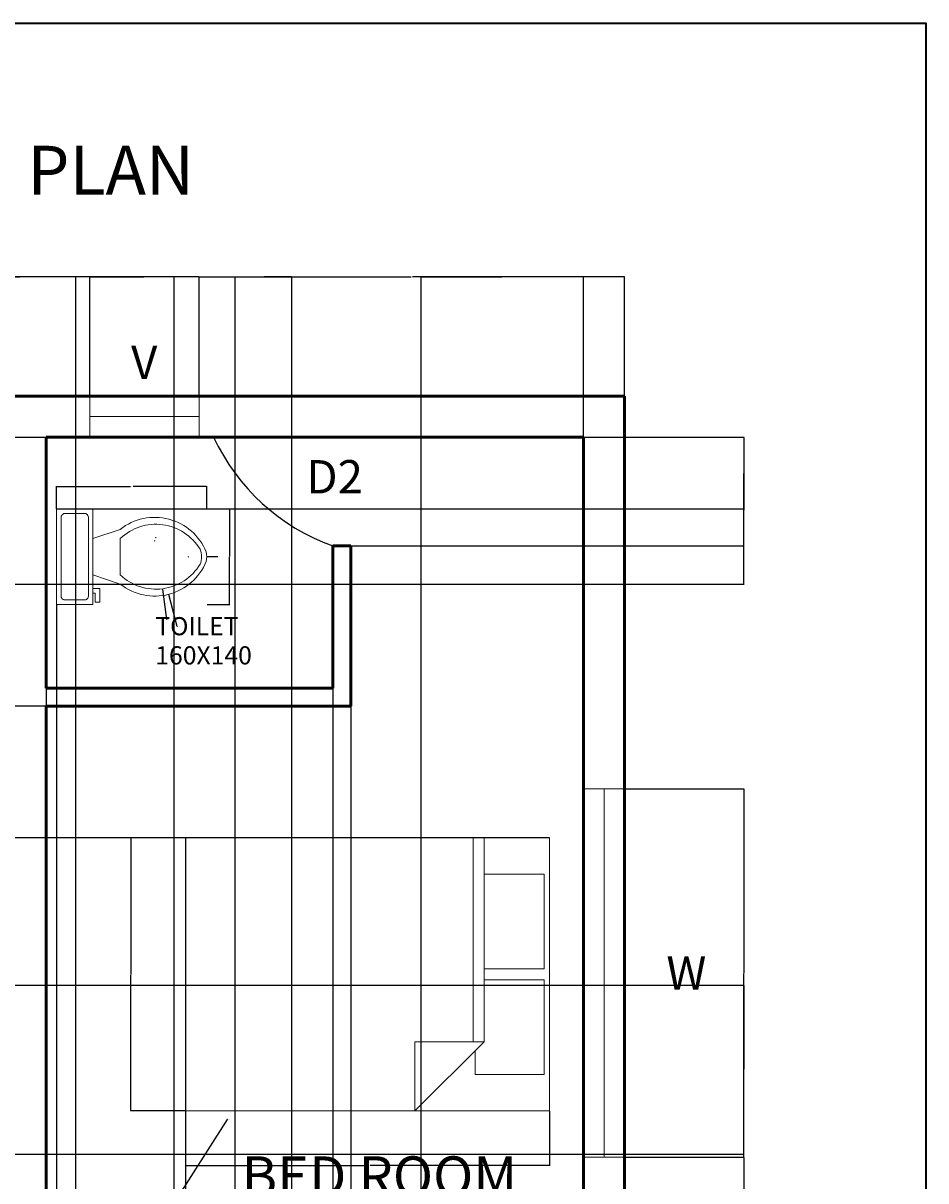
# Model space of a CAD drawing. Units: centimetres. Extents: x 2050 to 3144, y 831 to 2296.
# Tile 7 of 7: x 2640 to 3144, y 1650 to 2296. Entities that reach past the tile are written whole.
import ezdxf

# ---------------------------------------------------------------- set-up
doc = ezdxf.new("R2010")
doc.units = ezdxf.units.CM
for name, color, linetype, lineweight in [('A-ANNO-DIMS', 2, 'Continuous', 18), ('A-ANNO-TEXT', 7, 'Continuous', 18), ('A-ANNO-TTLB', 7, 'Continuous', 35), ('A-AREA-IDEN', 7, 'Continuous', 25), ('A-DOOR', 3, 'Continuous', 25), ('A-FLOR-FIXT', 8, 'Continuous', 18), ('A-FURN', 8, 'Continuous', 18), ('A-GLAZ', 4, 'Continuous', 18), ('A-WALL', 7, 'Continuous', 50)]:
    doc.layers.add(name, color=color, linetype=linetype, lineweight=lineweight)
doc.styles.get("Standard").update_dxf_attribs({"font": 'arial.ttf'})
doc.dimstyles.get("Standard").update_dxf_attribs({"dimtxt": 0.18, "dimasz": 0.18, "dimexe": 0.18, "dimexo": 0.0625, "dimgap": 0.09, "dimtad": 0, "dimtih": 1, "dimtoh": 1, "dimdec": 4, "dimzin": 0, "dimdsep": 46, "dimtxsty": 'Standard', "dimcen": 0.09, "dimadec": 0, "dimazin": 0, "dimtfac": 1, "dimtdec": 4, "dimtofl": 0, "dimtmove": 0, "dimatfit": 3, "dimfxl": 1, "dimtolj": 1, "dimtzin": 0, "dimarcsym": 0})

# ---------------------------------------------------------------- blocks, each defined once
blk = doc.blocks.new('Bed - Queen')
for p, q in [((0, -80.00003), (0, 0)), ((0, 0), (59.99999, 0)), ((59.99999, 0), (59.99999, -80.00003)), ((7.99999, -1.2), (28.79998, -1.2)), ((7.99999, -14.4), (7.99999, -1.2)), ((28.79998, -1.2), (28.79998, -14.4)), ((31.19999, -1.2), (51.99999, -1.2)), ((31.19999, -14.4), (31.19999, -1.2)), ((51.99999, -1.2), (51.99999, -16.4)), ((0, -14.4), (44.8, -14.4)), ((59.99999, -29.6), (44.8, -14.4)), ((44.8, -14.4), (44.8, -29.6)), ((44.8, -16.8), (0, -16.8)), ((51.99999, -16.4), (46.79936, -16.4)), ((44.8, -29.6), (59.99999, -29.6)), ((59.99999, -80.00003), (0, -80.00003))]:
    blk.add_line(p, q)
blk = doc.blocks.new('Toilet - top')
for p, q in [((9.5, -6), (9.5, -2)), ((-10, -8.5), (-8, -8.5)), ((-10, -9.5), (-10, -8.5)), ((-7, -9.5), (-10, -9.5)), ((-8, -8.5), (-8, -8)), ((-7, -8), (-7, -9.5)), ((-4, -8), (-6, -14)), ((4, -8), (6, -14)), ((4, -14), (-4, -14))]:
    blk.add_line(p, q)
blk.add_lwpolyline([(10.5, -8), (10.5, 0), (-10.5, 0), (-10.5, -8)], close=True)
for points in [[(-9.5, -2), (-9.5, -6)], [(8.5, -1), (-8.5, -1)], [(-8.5, -7), (8.5, -7)]]:
    blk.add_lwpolyline(points)
for centre, radius, start, end in [((-8.62, -1.88), 0.884, 81.8699, 188.1301), ((8.62, -1.88), 0.884, 351.8699, 98.1301), ((-8.62, -6.12), 0.884, 171.8699, 278.1301), ((8.62, -6.12), 0.884, 261.8699, 8.1301), ((3.52, -21.58), 12.17, 141.4691, 247.9714), ((4.2, -21.82), 11.33, 136.3677, 238.9468), ((-3.52, -21.58), 12.17, 292.0284, 38.5307), ((-4.2, -21.82), 11.33, 301.053, 43.6321), ((0, -27.88), 4, 245.7318, 294.2682), ((0, -29), 4, 254.8605, 285.1395)]:
    blk.add_arc(centre, radius, start, end)
blk = doc.blocks.new('*D11')
at = {"layer": 'A-ANNO-DIMS', "color": 0, "lineweight": -2, "transparency": 16777216}
for p, q in [((2730.58, 1688.9), (2730.58, 1658.3)), ((2933.78, 1688.9), (2933.78, 1658.3)), ((2730.76, 1658.48), (2830.81, 1658.48)), ((2933.6, 1658.48), (2833.55, 1658.48))]:
    blk.add_line(p, q, dxfattribs=at)
at = {"layer": 'A-ANNO-DIMS', "color": 0, "transparency": 16777216}
for points in [[(2730.76, 1658.51), (2730.76, 1658.45), (2730.58, 1658.48)], [(2933.6, 1658.51), (2933.6, 1658.45), (2933.78, 1658.48)]]:
    blk.add_solid(points, dxfattribs=at)
at = {"layer": 'Defpoints', "color": 0, "transparency": 16777216}
for p in [(2730.58, 1688.96), (2933.78, 1688.96), (2933.78, 1658.48)]:
    blk.add_point(p, dxfattribs=at)
at = {"layer": 'A-ANNO-DIMS', "color": 0, "transparency": 16777216, "insert": (2832.18, 1658.48), "char_height": 0.18, "attachment_point": 5}
blk.add_mtext('\\A1;QUEEN BED 203 TYP.', dxfattribs=at)
blk = doc.blocks.new('*D12')
at = {"layer": 'A-ANNO-DIMS', "color": 0, "lineweight": -2, "transparency": 16777216}
for p, q in [((2730.52, 1841.36), (2699.92, 1841.36)), ((2700.1, 1841.18), (2700.1, 1765.34)), ((2700.1, 1689.14), (2700.1, 1764.98)), ((2730.52, 1688.96), (2699.92, 1688.96))]:
    blk.add_line(p, q, dxfattribs=at)
at = {"layer": 'A-ANNO-DIMS', "color": 0, "transparency": 16777216}
for points in [[(2700.07, 1841.18), (2700.13, 1841.18), (2700.1, 1841.36)], [(2700.07, 1689.14), (2700.13, 1689.14), (2700.1, 1688.96)]]:
    blk.add_solid(points, dxfattribs=at)
at = {"layer": 'Defpoints', "color": 0, "transparency": 16777216}
for p in [(2730.58, 1841.36), (2700.1, 1688.96), (2730.58, 1688.96)]:
    blk.add_point(p, dxfattribs=at)
at = {"layer": 'A-ANNO-DIMS', "color": 0, "transparency": 16777216, "insert": (2700.1, 1765.16), "char_height": 0.18, "attachment_point": 5}
blk.add_mtext('\\A1;152 TYP.', dxfattribs=at)
blk = doc.blocks.new('*D13')
at = {"layer": 'A-ANNO-DIMS', "color": 0, "lineweight": -2, "transparency": 16777216}
for p, q in [((2658.57, 2024.91), (2658.57, 2037.62)), ((2658.75, 2037.44), (2699.77, 2037.44)), ((2742.33, 2037.44), (2701.32, 2037.44)), ((2742.51, 2024.91), (2742.51, 2037.62))]:
    blk.add_line(p, q, dxfattribs=at)
at = {"layer": 'A-ANNO-DIMS', "color": 0, "transparency": 16777216}
for points in [[(2658.75, 2037.47), (2658.75, 2037.41), (2658.57, 2037.44)], [(2742.33, 2037.47), (2742.33, 2037.41), (2742.51, 2037.44)]]:
    blk.add_solid(points, dxfattribs=at)
at = {"layer": 'Defpoints', "color": 0, "transparency": 16777216}
for p in [(2658.57, 2037.44), (2658.57, 2024.85), (2742.51, 2024.85)]:
    blk.add_point(p, dxfattribs=at)
at = {"layer": 'A-ANNO-DIMS', "color": 0, "transparency": 16777216, "insert": (2700.54, 2037.44), "char_height": 0.18, "attachment_point": 5}
blk.add_mtext('\\A1;WC 84 TYP.', dxfattribs=at)
blk = doc.blocks.new('*D14')
at = {"layer": 'A-ANNO-DIMS', "color": 0, "lineweight": -2, "transparency": 16777216}
for p, q in [((2742.57, 2024.85), (2755.28, 2024.85)), ((2755.1, 2024.67), (2755.1, 1998.36)), ((2755.1, 1971.69), (2755.1, 1998)), ((2742.57, 1971.51), (2755.28, 1971.51))]:
    blk.add_line(p, q, dxfattribs=at)
at = {"layer": 'A-ANNO-DIMS', "color": 0, "transparency": 16777216}
for points in [[(2755.07, 2024.67), (2755.13, 2024.67), (2755.1, 2024.85)], [(2755.07, 1971.69), (2755.13, 1971.69), (2755.1, 1971.51)]]:
    blk.add_solid(points, dxfattribs=at)
at = {"layer": 'Defpoints', "color": 0, "transparency": 16777216}
for p in [(2742.51, 2024.85), (2755.1, 2024.85), (2742.51, 1971.51)]:
    blk.add_point(p, dxfattribs=at)
at = {"layer": 'A-ANNO-DIMS', "color": 0, "transparency": 16777216, "insert": (2755.1, 1998.18), "char_height": 0.18, "attachment_point": 5}
blk.add_mtext('\\A1;53 TYP.', dxfattribs=at)
blk = doc.blocks.new('*D36')
at = {"layer": 'A-ANNO-DIMS', "color": 0, "lineweight": -2, "transparency": 16777216}
for p, q in [((2738.07, 2087.82), (2738.07, 2154.53)), ((2738.25, 2154.35), (2856.43, 2154.35)), ((2975.41, 2154.35), (2857.22, 2154.35)), ((2975.59, 2087.82), (2975.59, 2154.53))]:
    blk.add_line(p, q, dxfattribs=at)
at = {"layer": 'A-ANNO-DIMS', "color": 0, "transparency": 16777216}
for points in [[(2738.25, 2154.38), (2738.25, 2154.32), (2738.07, 2154.35)], [(2975.41, 2154.38), (2975.41, 2154.32), (2975.59, 2154.35)]]:
    blk.add_solid(points, dxfattribs=at)
at = {"layer": 'Defpoints', "color": 0, "transparency": 16777216}
for p in [(2975.59, 2154.35), (2738.07, 2087.75), (2975.59, 2087.75)]:
    blk.add_point(p, dxfattribs=at)
at = {"layer": 'A-ANNO-DIMS', "color": 0, "transparency": 16777216, "insert": (2856.83, 2154.35), "char_height": 0.18, "attachment_point": 5}
blk.add_mtext('\\A1;237.5', dxfattribs=at)
blk = doc.blocks.new('*D37')
at = {"layer": 'A-ANNO-DIMS', "color": 0, "lineweight": -2, "transparency": 16777216}
for p, q in [((2677.11, 2087.82), (2677.11, 2154.53)), ((2677.29, 2154.35), (2707.19, 2154.35)), ((2737.89, 2154.35), (2707.98, 2154.35)), ((2738.07, 2087.82), (2738.07, 2154.53))]:
    blk.add_line(p, q, dxfattribs=at)
at = {"layer": 'A-ANNO-DIMS', "color": 0, "transparency": 16777216}
for points in [[(2677.29, 2154.38), (2677.29, 2154.32), (2677.11, 2154.35)], [(2737.89, 2154.38), (2737.89, 2154.32), (2738.07, 2154.35)]]:
    blk.add_solid(points, dxfattribs=at)
at = {"layer": 'Defpoints', "color": 0, "transparency": 16777216}
for p in [(2738.07, 2154.35), (2677.11, 2087.75), (2738.07, 2087.75)]:
    blk.add_point(p, dxfattribs=at)
at = {"layer": 'A-ANNO-DIMS', "color": 0, "transparency": 16777216, "insert": (2707.59, 2154.35), "char_height": 0.18, "attachment_point": 5}
blk.add_mtext('\\A1;60.96', dxfattribs=at)
blk = doc.blocks.new('*D45')
at = {"layer": 'A-ANNO-DIMS', "color": 0, "lineweight": -2, "transparency": 16777216}
for p, q in [((2975.65, 1663.11), (3042.37, 1663.11)), ((3042.19, 1662.93), (3042.19, 1603.62)), ((3042.19, 1543.94), (3042.19, 1603.25)), ((2975.65, 1543.76), (3042.37, 1543.76))]:
    blk.add_line(p, q, dxfattribs=at)
at = {"layer": 'A-ANNO-DIMS', "color": 0, "transparency": 16777216}
for points in [[(3042.16, 1662.93), (3042.22, 1662.93), (3042.19, 1663.11)], [(3042.16, 1543.94), (3042.22, 1543.94), (3042.19, 1543.76)]]:
    blk.add_solid(points, dxfattribs=at)
at = {"layer": 'Defpoints', "color": 0, "transparency": 16777216}
for p in [(2975.59, 1663.11), (3042.19, 1663.11), (2975.59, 1543.76)]:
    blk.add_point(p, dxfattribs=at)
at = {"layer": 'A-ANNO-DIMS', "color": 0, "transparency": 16777216, "insert": (3042.19, 1603.43), "char_height": 0.18, "attachment_point": 5}
blk.add_mtext('\\A1;119.36', dxfattribs=at)
blk = doc.blocks.new('*D46')
at = {"layer": 'A-ANNO-DIMS', "color": 0, "lineweight": -2, "transparency": 16777216}
for p, q in [((2975.65, 1868.74), (3042.37, 1868.74)), ((3042.19, 1868.56), (3042.19, 1766.11)), ((3042.19, 1663.29), (3042.19, 1765.74)), ((2975.65, 1663.11), (3042.37, 1663.11))]:
    blk.add_line(p, q, dxfattribs=at)
at = {"layer": 'A-ANNO-DIMS', "color": 0, "transparency": 16777216}
for points in [[(3042.16, 1868.56), (3042.22, 1868.56), (3042.19, 1868.74)], [(3042.16, 1663.29), (3042.22, 1663.29), (3042.19, 1663.11)]]:
    blk.add_solid(points, dxfattribs=at)
at = {"layer": 'Defpoints', "color": 0, "transparency": 16777216}
for p in [(2975.59, 1868.74), (3042.19, 1868.74), (2975.59, 1663.11)]:
    blk.add_point(p, dxfattribs=at)
at = {"layer": 'A-ANNO-DIMS', "color": 0, "transparency": 16777216, "insert": (3042.19, 1765.92), "char_height": 0.18, "attachment_point": 5}
blk.add_mtext('\\A1;205.63', dxfattribs=at)
blk = doc.blocks.new('*D48')
at = {"layer": 'A-ANNO-DIMS', "color": 0, "lineweight": -2, "transparency": 16777216}
for p, q in [((2552.73, 1211.94), (2552.73, 2154.53)), ((2552.91, 2154.35), (2610.59, 2154.35)), ((2669.05, 2154.35), (2611.37, 2154.35)), ((2669.23, 1211.94), (2669.23, 2154.53))]:
    blk.add_line(p, q, dxfattribs=at)
at = {"layer": 'A-ANNO-DIMS', "color": 0, "transparency": 16777216}
for points in [[(2552.91, 2154.38), (2552.91, 2154.32), (2552.73, 2154.35)], [(2669.05, 2154.38), (2669.05, 2154.32), (2669.23, 2154.35)]]:
    blk.add_solid(points, dxfattribs=at)
at = {"layer": 'Defpoints', "color": 0, "transparency": 16777216}
for p in [(2669.23, 2154.35), (2552.73, 1211.87), (2669.23, 1211.87)]:
    blk.add_point(p, dxfattribs=at)
at = {"layer": 'A-ANNO-DIMS', "color": 0, "transparency": 16777216, "insert": (2610.98, 2154.35), "char_height": 0.18, "attachment_point": 5}
blk.add_mtext('\\A1;116.5', dxfattribs=at)
blk = doc.blocks.new('*D54')
at = {"layer": 'A-ANNO-DIMS', "color": 0, "lineweight": -2, "transparency": 16777216}
for p, q in [((2515.69, 2064.89), (3042.37, 2064.89)), ((3042.19, 2064.71), (3042.19, 2024.09)), ((3042.19, 1983.1), (3042.19, 2023.73)), ((2515.69, 1982.92), (3042.37, 1982.92))]:
    blk.add_line(p, q, dxfattribs=at)
at = {"layer": 'A-ANNO-DIMS', "color": 0, "transparency": 16777216}
for points in [[(3042.16, 2064.71), (3042.22, 2064.71), (3042.19, 2064.89)], [(3042.16, 1983.1), (3042.22, 1983.1), (3042.19, 1982.92)]]:
    blk.add_solid(points, dxfattribs=at)
at = {"layer": 'Defpoints', "color": 0, "transparency": 16777216}
for p in [(2515.63, 2064.89), (3042.19, 2064.89), (2515.63, 1982.92)]:
    blk.add_point(p, dxfattribs=at)
at = {"layer": 'A-ANNO-DIMS', "color": 0, "transparency": 16777216, "insert": (3042.19, 2023.91), "char_height": 0.18, "attachment_point": 5}
blk.add_mtext('\\A1;81.97', dxfattribs=at)
blk = doc.blocks.new('*D55')
at = {"layer": 'A-ANNO-DIMS', "color": 0, "lineweight": -2, "transparency": 16777216}
for p, q in [((2822.95, 2064.89), (3042.37, 2064.89)), ((3042.19, 2064.71), (3042.19, 2034.74)), ((3042.19, 2004.4), (3042.19, 2034.38)), ((2812.79, 2004.22), (3042.37, 2004.22))]:
    blk.add_line(p, q, dxfattribs=at)
at = {"layer": 'A-ANNO-DIMS', "color": 0, "transparency": 16777216}
for points in [[(3042.16, 2064.71), (3042.22, 2064.71), (3042.19, 2064.89)], [(3042.16, 2004.4), (3042.22, 2004.4), (3042.19, 2004.22)]]:
    blk.add_solid(points, dxfattribs=at)
at = {"layer": 'Defpoints', "color": 0, "transparency": 16777216}
for p in [(2822.89, 2064.89), (3042.19, 2064.89), (2812.73, 2004.22)]:
    blk.add_point(p, dxfattribs=at)
at = {"layer": 'A-ANNO-DIMS', "color": 0, "transparency": 16777216, "insert": (3042.19, 2034.56), "char_height": 0.18, "attachment_point": 5}
blk.add_mtext('\\A1;60.67', dxfattribs=at)
blk = doc.blocks.new('*D59')
at = {"layer": 'A-ANNO-DIMS', "color": 0, "lineweight": -2, "transparency": 16777216}
for p, q in [((2862.15, 1253.11), (2862.15, 2154.53)), ((2862.33, 2154.35), (2907.04, 2154.35)), ((2952.55, 2154.35), (2907.83, 2154.35)), ((2952.73, 1211.94), (2952.73, 2154.53))]:
    blk.add_line(p, q, dxfattribs=at)
at = {"layer": 'A-ANNO-DIMS', "color": 0, "transparency": 16777216}
for points in [[(2862.33, 2154.38), (2862.33, 2154.32), (2862.15, 2154.35)], [(2952.55, 2154.38), (2952.55, 2154.32), (2952.73, 2154.35)]]:
    blk.add_solid(points, dxfattribs=at)
at = {"layer": 'Defpoints', "color": 0, "transparency": 16777216}
for p in [(2952.73, 2154.35), (2862.15, 1253.05), (2952.73, 1211.87)]:
    blk.add_point(p, dxfattribs=at)
at = {"layer": 'A-ANNO-DIMS', "color": 0, "transparency": 16777216, "insert": (2907.44, 2154.35), "char_height": 0.18, "attachment_point": 5}
blk.add_mtext('\\A1;90.58', dxfattribs=at)
blk = doc.blocks.new('*D61')
at = {"layer": 'A-ANNO-DIMS', "color": 0, "lineweight": -2, "transparency": 16777216}
for p, q in [((2552.73, 1328.44), (2552.73, 2154.53)), ((2552.91, 2154.35), (2638.04, 2154.35)), ((2723.95, 2154.35), (2638.81, 2154.35)), ((2724.13, 1334.5), (2724.13, 2154.53))]:
    blk.add_line(p, q, dxfattribs=at)
at = {"layer": 'A-ANNO-DIMS', "color": 0, "transparency": 16777216}
for points in [[(2552.91, 2154.38), (2552.91, 2154.32), (2552.73, 2154.35)], [(2723.95, 2154.38), (2723.95, 2154.32), (2724.13, 2154.35)]]:
    blk.add_solid(points, dxfattribs=at)
at = {"layer": 'Defpoints', "color": 0, "transparency": 16777216}
for p in [(2724.13, 2154.35), (2724.13, 1334.43), (2552.73, 1328.38)]:
    blk.add_point(p, dxfattribs=at)
at = {"layer": 'A-ANNO-DIMS', "color": 0, "transparency": 16777216, "insert": (2638.43, 2154.35), "char_height": 0.18, "attachment_point": 5}
blk.add_mtext('\\A1;171.4', dxfattribs=at)
blk = doc.blocks.new('*D62')
at = {"layer": 'A-ANNO-DIMS', "color": 0, "lineweight": -2, "transparency": 16777216}
for p, q in [((2758.2, 1334.5), (2758.2, 2154.53)), ((2758.38, 2154.35), (2773.58, 2154.35)), ((2789.71, 2154.35), (2774.51, 2154.35)), ((2789.89, 1319.12), (2789.89, 2154.53))]:
    blk.add_line(p, q, dxfattribs=at)
at = {"layer": 'A-ANNO-DIMS', "color": 0, "transparency": 16777216}
for points in [[(2758.38, 2154.38), (2758.38, 2154.32), (2758.2, 2154.35)], [(2789.71, 2154.38), (2789.71, 2154.32), (2789.89, 2154.35)]]:
    blk.add_solid(points, dxfattribs=at)
at = {"layer": 'Defpoints', "color": 0, "transparency": 16777216}
for p in [(2789.89, 2154.35), (2758.2, 1334.43), (2789.89, 1319.06)]:
    blk.add_point(p, dxfattribs=at)
at = {"layer": 'A-ANNO-DIMS', "color": 0, "transparency": 16777216, "insert": (2774.05, 2154.35), "char_height": 0.18, "attachment_point": 5}
blk.add_mtext('\\A1;31.696', dxfattribs=at)
blk = doc.blocks.new('*D65')
at = {"layer": 'A-ANNO-DIMS', "color": 0, "lineweight": -2, "transparency": 16777216}
for p, q in [((2812.73, 1924.83), (2812.73, 1009.53)), ((2822.89, 1914.67), (2822.89, 1009.53)), ((2812.91, 1009.71), (2817.42, 1009.71)), ((2822.71, 1009.71), (2818.19, 1009.71))]:
    blk.add_line(p, q, dxfattribs=at)
at = {"layer": 'A-ANNO-DIMS', "color": 0, "transparency": 16777216}
for points in [[(2812.91, 1009.74), (2812.91, 1009.68), (2812.73, 1009.71)], [(2822.71, 1009.74), (2822.71, 1009.68), (2822.89, 1009.71)]]:
    blk.add_solid(points, dxfattribs=at)
at = {"layer": 'Defpoints', "color": 0, "transparency": 16777216}
for p in [(2812.73, 1924.89), (2822.89, 1914.73), (2822.89, 1009.71)]:
    blk.add_point(p, dxfattribs=at)
at = {"layer": 'A-ANNO-DIMS', "color": 0, "transparency": 16777216, "insert": (2817.81, 1009.71), "char_height": 0.18, "attachment_point": 5}
blk.add_mtext('\\A1;10.16', dxfattribs=at)
blk = doc.blocks.new('*D68')
at = {"layer": 'A-ANNO-DIMS', "color": 0, "lineweight": -2, "transparency": 16777216}
for p, q in [((2652.73, 1914.67), (2652.73, 1009.53)), ((2730.58, 1841.3), (2730.58, 1009.53)), ((2652.91, 1009.71), (2691.26, 1009.71)), ((2730.4, 1009.71), (2692.05, 1009.71))]:
    blk.add_line(p, q, dxfattribs=at)
at = {"layer": 'A-ANNO-DIMS', "color": 0, "transparency": 16777216}
for points in [[(2652.91, 1009.74), (2652.91, 1009.68), (2652.73, 1009.71)], [(2730.4, 1009.74), (2730.4, 1009.68), (2730.58, 1009.71)]]:
    blk.add_solid(points, dxfattribs=at)
at = {"layer": 'Defpoints', "color": 0, "transparency": 16777216}
for p in [(2652.73, 1914.73), (2730.58, 1841.36), (2730.58, 1009.71)]:
    blk.add_point(p, dxfattribs=at)
at = {"layer": 'A-ANNO-DIMS', "color": 0, "transparency": 16777216, "insert": (2691.65, 1009.71), "char_height": 0.18, "attachment_point": 5}
blk.add_mtext('\\A1;77.85', dxfattribs=at)
blk = doc.blocks.new('*D69')
at = {"layer": 'A-ANNO-DIMS', "color": 0, "lineweight": -2, "transparency": 16777216}
for p, q in [((2822.82, 1914.73), (2120.23, 1914.73)), ((2120.41, 1914.55), (2120.41, 1878.23)), ((2120.41, 1841.54), (2120.41, 1877.86)), ((2933.72, 1841.36), (2120.23, 1841.36))]:
    blk.add_line(p, q, dxfattribs=at)
at = {"layer": 'A-ANNO-DIMS', "color": 0, "transparency": 16777216}
for points in [[(2120.38, 1914.55), (2120.44, 1914.55), (2120.41, 1914.73)], [(2120.38, 1841.54), (2120.44, 1841.54), (2120.41, 1841.36)]]:
    blk.add_solid(points, dxfattribs=at)
at = {"layer": 'Defpoints', "color": 0, "transparency": 16777216}
for p in [(2120.41, 1914.73), (2822.89, 1914.73), (2933.78, 1841.36)]:
    blk.add_point(p, dxfattribs=at)
at = {"layer": 'A-ANNO-DIMS', "color": 0, "transparency": 16777216, "insert": (2120.41, 1878.05), "char_height": 0.18, "attachment_point": 5}
blk.add_mtext('\\A1;73.38', dxfattribs=at)
blk = doc.blocks.new('*D71')
at = {"layer": 'A-ANNO-DIMS', "color": 0, "lineweight": -2, "transparency": 16777216}
for p, q in [((2219.88, 1759.22), (3042.37, 1759.22)), ((3042.19, 1759.04), (3042.19, 1712.24)), ((3042.19, 1665.07), (3042.19, 1711.88)), ((2209.93, 1664.89), (3042.37, 1664.89))]:
    blk.add_line(p, q, dxfattribs=at)
at = {"layer": 'A-ANNO-DIMS', "color": 0, "transparency": 16777216}
for points in [[(3042.16, 1759.04), (3042.22, 1759.04), (3042.19, 1759.22)], [(3042.16, 1665.07), (3042.22, 1665.07), (3042.19, 1664.89)]]:
    blk.add_solid(points, dxfattribs=at)
at = {"layer": 'Defpoints', "color": 0, "transparency": 16777216}
for p in [(2219.81, 1759.22), (3042.19, 1759.22), (2209.87, 1664.89)]:
    blk.add_point(p, dxfattribs=at)
at = {"layer": 'A-ANNO-DIMS', "color": 0, "transparency": 16777216, "insert": (3042.19, 1712.06), "char_height": 0.18, "attachment_point": 5}
blk.add_mtext('\\A1;94.33', dxfattribs=at)
blk = doc.blocks.new('*D72')
at = {"layer": 'A-ANNO-DIMS', "color": 0, "lineweight": -2, "transparency": 16777216}
for p, q in [((2652.79, 2064.89), (3042.37, 2064.89)), ((3042.19, 2064.71), (3042.19, 2045.06)), ((3042.19, 2025.03), (3042.19, 2044.69)), ((2658.64, 2024.85), (3042.37, 2024.85))]:
    blk.add_line(p, q, dxfattribs=at)
at = {"layer": 'A-ANNO-DIMS', "color": 0, "transparency": 16777216}
for points in [[(3042.16, 2064.71), (3042.22, 2064.71), (3042.19, 2064.89)], [(3042.16, 2025.03), (3042.22, 2025.03), (3042.19, 2024.85)]]:
    blk.add_solid(points, dxfattribs=at)
at = {"layer": 'Defpoints', "color": 0, "transparency": 16777216}
for p in [(2652.73, 2064.89), (2658.57, 2024.85), (3042.19, 2024.85)]:
    blk.add_point(p, dxfattribs=at)
at = {"layer": 'A-ANNO-DIMS', "color": 0, "transparency": 16777216, "insert": (3042.19, 2044.87), "char_height": 0.18, "attachment_point": 5}
blk.add_mtext('\\A1;40.04', dxfattribs=at)
blk = doc.blocks.new('*D73')
at = {"layer": 'A-ANNO-DIMS', "color": 0, "lineweight": -2, "transparency": 16777216}
for p, q in [((2658.57, 1971.45), (2658.57, 1009.53)), ((2652.73, 1924.83), (2652.73, 1009.53)), ((2652.91, 1009.71), (2655.26, 1009.71)), ((2658.39, 1009.71), (2656.04, 1009.71))]:
    blk.add_line(p, q, dxfattribs=at)
at = {"layer": 'A-ANNO-DIMS', "color": 0, "transparency": 16777216}
for points in [[(2652.91, 1009.74), (2652.91, 1009.68), (2652.73, 1009.71)], [(2658.39, 1009.74), (2658.39, 1009.68), (2658.57, 1009.71)]]:
    blk.add_solid(points, dxfattribs=at)
at = {"layer": 'Defpoints', "color": 0, "transparency": 16777216}
for p in [(2658.57, 1971.51), (2652.73, 1924.89), (2658.57, 1009.71)]:
    blk.add_point(p, dxfattribs=at)
at = {"layer": 'A-ANNO-DIMS', "color": 0, "transparency": 16777216, "insert": (2655.65, 1009.71), "char_height": 0.18, "attachment_point": 5}
blk.add_mtext('\\A1;5.847', dxfattribs=at)
blk = doc.blocks.new('*D74')
at = {"layer": 'A-ANNO-DIMS', "color": 0, "lineweight": -2, "transparency": 16777216}
for p, q in [((2952.73, 2064.83), (2952.73, 1009.53)), ((2822.89, 2004.16), (2822.89, 1009.53)), ((2823.07, 1009.71), (2887.35, 1009.71)), ((2952.55, 1009.71), (2888.26, 1009.71))]:
    blk.add_line(p, q, dxfattribs=at)
at = {"layer": 'A-ANNO-DIMS', "color": 0, "transparency": 16777216}
for points in [[(2823.07, 1009.74), (2823.07, 1009.68), (2822.89, 1009.71)], [(2952.55, 1009.74), (2952.55, 1009.68), (2952.73, 1009.71)]]:
    blk.add_solid(points, dxfattribs=at)
at = {"layer": 'Defpoints', "color": 0, "transparency": 16777216}
for p in [(2952.73, 2064.89), (2822.89, 2004.22), (2952.73, 1009.71)]:
    blk.add_point(p, dxfattribs=at)
at = {"layer": 'A-ANNO-DIMS', "color": 0, "transparency": 16777216, "insert": (2887.81, 1009.71), "char_height": 0.18, "attachment_point": 5}
blk.add_mtext('\\A1;129.84', dxfattribs=at)
blk = doc.blocks.new('*D76')
at = {"layer": 'A-ANNO-DIMS', "color": 0, "lineweight": -2, "transparency": 16777216}
for p, q in [((2753.78, 1684.12), (2714.94, 1623.27)), ((2753.96, 1684.12), (2753.78, 1684.12)), ((2649.86, 1521.45), (2650.04, 1521.45)), ((2649.95, 1521.36), (2649.95, 1521.54))]:
    blk.add_line(p, q, dxfattribs=at)
at = {"layer": 'A-ANNO-DIMS', "color": 0, "transparency": 16777216}
blk.add_solid([(2714.92, 1623.29), (2714.97, 1623.25), (2714.85, 1623.12)], dxfattribs=at)
at = {"layer": 'Defpoints', "color": 0, "transparency": 16777216}
for p in [(2714.85, 1623.12), (2649.95, 1521.45)]:
    blk.add_point(p, dxfattribs=at)
at = {"layer": 'A-ANNO-DIMS', "color": 0, "transparency": 16777216, "insert": (2754.5, 1684.12), "char_height": 0.18, "attachment_point": 5}
blk.add_mtext('\\A1;R120.61', dxfattribs=at)
blk = doc.blocks.new('*D82')
at = {"layer": 'A-ANNO-DIMS', "color": 0, "lineweight": -2, "transparency": 16777216}
for p, q in [((2713.3, 2007.12), (2713.48, 2007.12)), ((2713.39, 2007.03), (2713.39, 2007.21)), ((2725.95, 1959.29), (2721.29, 1977.05)), ((2726.13, 1959.29), (2725.95, 1959.29))]:
    blk.add_line(p, q, dxfattribs=at)
at = {"layer": 'A-ANNO-DIMS', "color": 0, "transparency": 16777216}
blk.add_solid([(2721.32, 1977.06), (2721.26, 1977.04), (2721.24, 1977.23)], dxfattribs=at)
at = {"layer": 'Defpoints', "color": 0, "transparency": 16777216}
for p in [(2713.39, 2007.12), (2721.24, 1977.23)]:
    blk.add_point(p, dxfattribs=at)
at = {"layer": 'A-ANNO-DIMS', "color": 0, "transparency": 16777216, "insert": (2726.79, 1959.29), "char_height": 0.18, "attachment_point": 5}
blk.add_mtext('\\A1;4X R30.91', dxfattribs=at)
blk = doc.blocks.new('*D83')
at = {"layer": 'A-ANNO-DIMS', "color": 0, "lineweight": -2, "transparency": 16777216}
for p, q in [((2713.9, 2008.85), (2714.08, 2008.85)), ((2713.99, 2008.76), (2713.99, 2008.94)), ((2720.12, 1963.22), (2717.85, 1980.15)), ((2720.3, 1963.22), (2720.12, 1963.22))]:
    blk.add_line(p, q, dxfattribs=at)
at = {"layer": 'A-ANNO-DIMS', "color": 0, "transparency": 16777216}
blk.add_solid([(2717.88, 1980.16), (2717.82, 1980.15), (2717.82, 1980.33)], dxfattribs=at)
at = {"layer": 'Defpoints', "color": 0, "transparency": 16777216}
for p in [(2713.99, 2008.85), (2717.82, 1980.33)]:
    blk.add_point(p, dxfattribs=at)
at = {"layer": 'A-ANNO-DIMS', "color": 0, "transparency": 16777216, "insert": (2721.05, 1963.22), "char_height": 0.18, "attachment_point": 5}
blk.add_mtext('\\A1;4X R28.776', dxfattribs=at)
blk = doc.blocks.new('*D84')
at = {"layer": 'A-ANNO-DIMS', "color": 0, "lineweight": -2, "transparency": 16777216}
for p, q in [((2732.14, 1998.18), (2732.32, 1998.18)), ((2732.23, 1998.09), (2732.23, 1998.27)), ((2748.49, 1998.18), (2742.57, 1998.18))]:
    blk.add_line(p, q, dxfattribs=at)
at = {"layer": 'A-ANNO-DIMS', "color": 0, "transparency": 16777216}
blk.add_solid([(2742.57, 1998.21), (2742.57, 1998.15), (2742.39, 1998.18)], dxfattribs=at)
at = {"layer": 'Defpoints', "color": 0, "transparency": 16777216}
for p in [(2732.23, 1998.18), (2742.39, 1998.18)]:
    blk.add_point(p, dxfattribs=at)
at = {"layer": 'A-ANNO-DIMS', "color": 0, "transparency": 16777216, "insert": (2749.17, 1998.18), "char_height": 0.18, "attachment_point": 5}
blk.add_mtext('\\A1;4X R10.16', dxfattribs=at)

msp = doc.modelspace()

# ---------------------------------------------------------------- linework, layer by layer
at = {"layer": 'A-ANNO-TTLB'}
msp.add_lwpolyline([(2050.3641, 2295.8578), (3143.7558, 2295.8578), (3143.7558, 830.6902), (2050.3641, 830.6902)], close=True, dxfattribs=at)
at = {"layer": 'A-DOOR'}
msp.add_line((2683.5212, 2064.8948), (2822.8865, 2064.8948), dxfattribs=at)
msp.add_arc((2851.9284, 2113.9321), 116.5053, 204.8915536, 250.3373359, dxfattribs=at)
at = {"layer": 'A-GLAZ'}
for p, q in [((2677.1054, 2087.7548), (2677.1054, 2064.8948)), ((2738.0654, 2087.7548), (2738.0654, 2064.8948)), ((2677.1054, 2076.3248), (2738.0654, 2076.3248)), ((2952.7265, 1868.738), (2975.5865, 1868.738)), ((2964.1565, 1868.738), (2964.1565, 1663.1111)), ((2952.7265, 1663.1111), (2975.5865, 1663.1111))]:
    msp.add_line(p, q, dxfattribs=at)
at = {"layer": 'A-WALL'}
for p, q in [((2629.8665, 2087.7548), (2975.5865, 2087.7548)), ((2652.7265, 2087.7548), (2975.5865, 2087.7548)), ((2975.5865, 2087.7548), (2975.5865, 1914.7348)), ((2652.7265, 2064.8948), (2652.7265, 1924.8948)), ((2652.7265, 2064.8948), (2952.7265, 2064.8948)), ((2952.7265, 2064.8948), (2952.7265, 1914.7348)), ((2812.7265, 2004.2202), (2812.7265, 1924.8948)), ((2812.7265, 2004.2202), (2822.8865, 2004.2202)), ((2822.8865, 1950.6542), (2822.8865, 2004.2202)), ((2822.8865, 2001.1046), (2822.8865, 1914.7348)), ((2812.7265, 1924.8948), (2652.7265, 1924.8948)), ((2822.8865, 1914.7348), (2652.7265, 1914.7348)), ((2652.7265, 1914.7348), (2652.7265, 1642.0348)), ((2952.7265, 1914.7348), (2952.7265, 1574.7348)), ((2975.5865, 1914.7348), (2975.5865, 1189.0148))]:
    msp.add_line(p, q, dxfattribs=at)

# ---------------------------------------------------------------- block references
at = {"layer": 'A-FLOR-FIXT', "xscale": 2.54, "yscale": 2.54, "zscale": 2.54, "rotation": 90}
msp.add_blockref('Toilet - top', (2658.5737, 1998.1818), dxfattribs=at)
at = {"layer": 'A-FURN', "xscale": 2.54, "yscale": 2.54, "zscale": 2.54, "rotation": 270}
msp.add_blockref('Bed - Queen', (2933.7791, 1841.3577), dxfattribs=at)

# ---------------------------------------------------------------- texts
at = {"layer": 'A-ANNO-TEXT'}
for s, height, p in [('V', 18.5959, (2700.1838, 2097.2451)), ('D2', 18.59595, (2798.0014, 2033.496)), ('W', 18.5959, (2998.9426, 1756.5453))]:
    msp.add_text(s, height=height, dxfattribs=at).set_placement(p)
at = {"layer": 'A-ANNO-TTLB'}
msp.add_text('2BHK HOUSE PLAN', height=27.192544, dxfattribs=at).set_placement((2404.4801, 2200.2444))
at = {"layer": 'A-AREA-IDEN'}
for s, height, p in [('TOILET', 10.12455, (2713.6552, 1954.3581)), ('160X140', 10.12455, (2713.6552, 1938.0939)), ('BED ROOM', 22.16939, (2761.802, 1641.4722))]:
    msp.add_text(s, height=height, dxfattribs=at).set_placement(p)

# ---------------------------------------------------------------- dimensions: what is measured, and where the dimension line sits
at = {"layer": 'A-ANNO-DIMS'}
for base, p1, p2, override, picture, middle in [((2669.2319, 2154.3548), (2552.7265, 1211.8748), (2669.2319, 1211.8748), {"dimdec": 1, "dimlfac": 1, "dimrnd": 0, "dimzin": 0, "dimdsep": 46, "dimlunit": 2}, '*D48', (2610.9792, 2154.3548)), ((2724.1318, 2154.3548), (2552.7265, 1328.3801), (2724.1318, 1334.433), {"dimdec": 1, "dimlfac": 1, "dimrnd": 0, "dimzin": 0, "dimdsep": 46, "dimlunit": 2}, '*D61', (2638.4292, 2154.3548)), ((2738.0654, 2154.3548), (2677.1054, 2087.7548), (2738.0654, 2087.7548), {"dimdec": 2, "dimlfac": 1, "dimrnd": 0, "dimzin": 0, "dimdsep": 46, "dimlunit": 2}, '*D37', (2707.5854, 2154.3548)), ((2975.5865, 2154.3548), (2738.0654, 2087.7548), (2975.5865, 2087.7548), {"dimdec": 1, "dimlfac": 1, "dimrnd": 0, "dimzin": 0, "dimdsep": 46, "dimlunit": 2}, '*D36', (2856.826, 2154.3548)), ((2789.8945, 2154.3548), (2758.1988, 1334.433), (2789.8945, 1319.0567), {"dimdec": 3, "dimlfac": 1, "dimrnd": 0, "dimzin": 0, "dimdsep": 46, "dimlunit": 2}, '*D62', (2774.0467, 2154.3548)), ((2952.7265, 2154.3548), (2862.1454, 1253.0515), (2952.7265, 1211.8748), {"dimdec": 2, "dimlfac": 1, "dimrnd": 0, "dimzin": 0, "dimdsep": 46, "dimlunit": 2}, '*D59', (2907.436, 2154.3548)), ((2952.7265, 1009.7148), (2822.8865, 2004.2202), (2952.7265, 2064.8948), {"dimdec": 2, "dimlfac": 1, "dimrnd": 0, "dimzin": 0, "dimdsep": 46, "dimlunit": 2}, '*D74', (2887.8065, 1009.7148)), ((2658.5737, 1009.7148), (2652.7265, 1924.8948), (2658.5737, 1971.5118), {"dimdec": 3, "dimlfac": 1, "dimrnd": 0, "dimzin": 0, "dimdsep": 46, "dimlunit": 2}, '*D73', (2655.6501, 1009.7148)), ((2822.8865, 1009.7148), (2812.7265, 1924.8948), (2822.8865, 1914.7348), {"dimdec": 2, "dimlfac": 1, "dimrnd": 0, "dimzin": 0, "dimdsep": 46, "dimlunit": 2}, '*D65', (2817.8065, 1009.7148)), ((2730.579, 1009.7148), (2652.7265, 1914.7348), (2730.579, 1841.3577), {"dimdec": 2, "dimlfac": 1, "dimrnd": 0, "dimzin": 0, "dimdsep": 46, "dimlunit": 2}, '*D68', (2691.6528, 1009.7148))]:
    dim = msp.add_linear_dim(base=base, p1=p1, p2=p2, dimstyle='Standard', override=override, dxfattribs=at)
    dim.commit()
    dim.dimension.update_dxf_attribs({"geometry": picture, "text_midpoint": middle})
for base, p1, p2, picture, middle in [((3042.1865, 2064.8948), (2515.6259, 1982.92), (2515.6259, 2064.8948), '*D54', (3042.1865, 2023.9074)), ((3042.1865, 2024.8518), (2652.7265, 2064.8948), (2658.5737, 2024.8518), '*D72', (3042.1865, 2044.8733)), ((3042.1865, 2064.8948), (2812.7265, 2004.2202), (2822.8865, 2064.8948), '*D55', (3042.1865, 2034.5575)), ((2120.4065, 1914.7348), (2933.7791, 1841.3577), (2822.8865, 1914.7348), '*D69', (2120.4065, 1878.0462)), ((3042.1865, 1868.738), (2975.5865, 1663.1111), (2975.5865, 1868.738), '*D46', (3042.1865, 1765.9245)), ((3042.1865, 1759.2218), (2209.8665, 1664.8948), (2219.8135, 1759.2218), '*D71', (3042.1865, 1712.0583)), ((3042.1865, 1663.1111), (2975.5865, 1543.7558), (2975.5865, 1663.1111), '*D45', (3042.1865, 1603.4335))]:
    dim = msp.add_linear_dim(base=base, p1=p1, p2=p2, angle=90, dimstyle='Standard', override={"dimdec": 2, "dimlfac": 1, "dimrnd": 0, "dimzin": 0, "dimdsep": 46, "dimlunit": 2}, dxfattribs=at)
    dim.commit()
    dim.dimension.update_dxf_attribs({"geometry": picture, "text_midpoint": middle})
for base, p1, p2, angle, text, picture, middle in [((2658.5737, 2037.4424), (2742.5112, 2024.8518), (2658.5737, 2024.8518), 180, 'WC <> TYP.', '*D13', (2700.5424, 2037.4424)), ((2755.1018, 2024.8518), (2742.5112, 1971.5118), (2742.5112, 2024.8518), 90, '<> TYP.', '*D14', (2755.1018, 1998.1818)), ((2700.099, 1688.9577), (2730.579, 1841.3577), (2730.579, 1688.9577), 270, '<> TYP.', '*D12', (2700.099, 1765.1577))]:
    dim = msp.add_linear_dim(base=base, p1=p1, p2=p2, angle=angle, text=text, dimstyle='Standard', override={"dimdec": 0, "dimlfac": 1, "dimrnd": 0, "dimzin": 0, "dimdsep": 46, "dimlunit": 2}, dxfattribs=at)
    dim.commit()
    dim.dimension.update_dxf_attribs({"geometry": picture, "text_midpoint": middle})
for center, mpoint, override, picture, middle in [((2713.9899, 2008.8497), (2717.824, 1980.3302), {"dimdec": 3, "dimlfac": 1, "dimrnd": 0, "dimzin": 0, "dimdsep": 46, "dimlunit": 2}, '*D83', (2721.0511, 1963.2184)), ((2713.3882, 2007.1215), (2721.2421, 1977.2267), {"dimdec": 2, "dimlfac": 1, "dimrnd": 0, "dimzin": 0, "dimdsep": 46, "dimlunit": 2}, '*D82', (2726.7939, 1959.2898)), ((2732.2336, 1998.1819), (2742.3936, 1998.182), {"dimdec": 2, "dimlfac": 1, "dimrnd": 0, "dimzin": 0, "dimdsep": 46, "dimlunit": 2}, '*D84', (2748.4896, 1998.1821))]:
    dim = msp.add_radius_dim(center=center, mpoint=mpoint, text='4X <>', dimstyle='Standard', override=override, dxfattribs=at)
    dim.commit()
    dim.dimension.update_dxf_attribs({"geometry": picture, "text_midpoint": middle, "dimtype": 164})
dim = msp.add_linear_dim(base=(2933.7791, 1658.4777), p1=(2730.579, 1688.9577), p2=(2933.7791, 1688.9577), text='QUEEN BED <> TYP.', dimstyle='Standard', override={"dimdec": 0, "dimlfac": 1, "dimrnd": 0, "dimzin": 0, "dimdsep": 46, "dimlunit": 2}, dxfattribs=at)
dim.commit()
dim.dimension.update_dxf_attribs({"geometry": '*D11', "text_midpoint": (2832.179, 1658.4777)})
dim = msp.add_radius_dim(center=(2649.9472, 1521.4533), mpoint=(2714.8457, 1623.1185), dimstyle='Standard', override={"dimdec": 2, "dimlfac": 1, "dimrnd": 0, "dimzin": 0, "dimdsep": 46, "dimlunit": 2}, dxfattribs=at)
dim.commit()
dim.dimension.update_dxf_attribs({"geometry": '*D76', "text_midpoint": (2754.4971, 1684.1176), "dimtype": 164})

doc.saveas('drawing.dxf')
